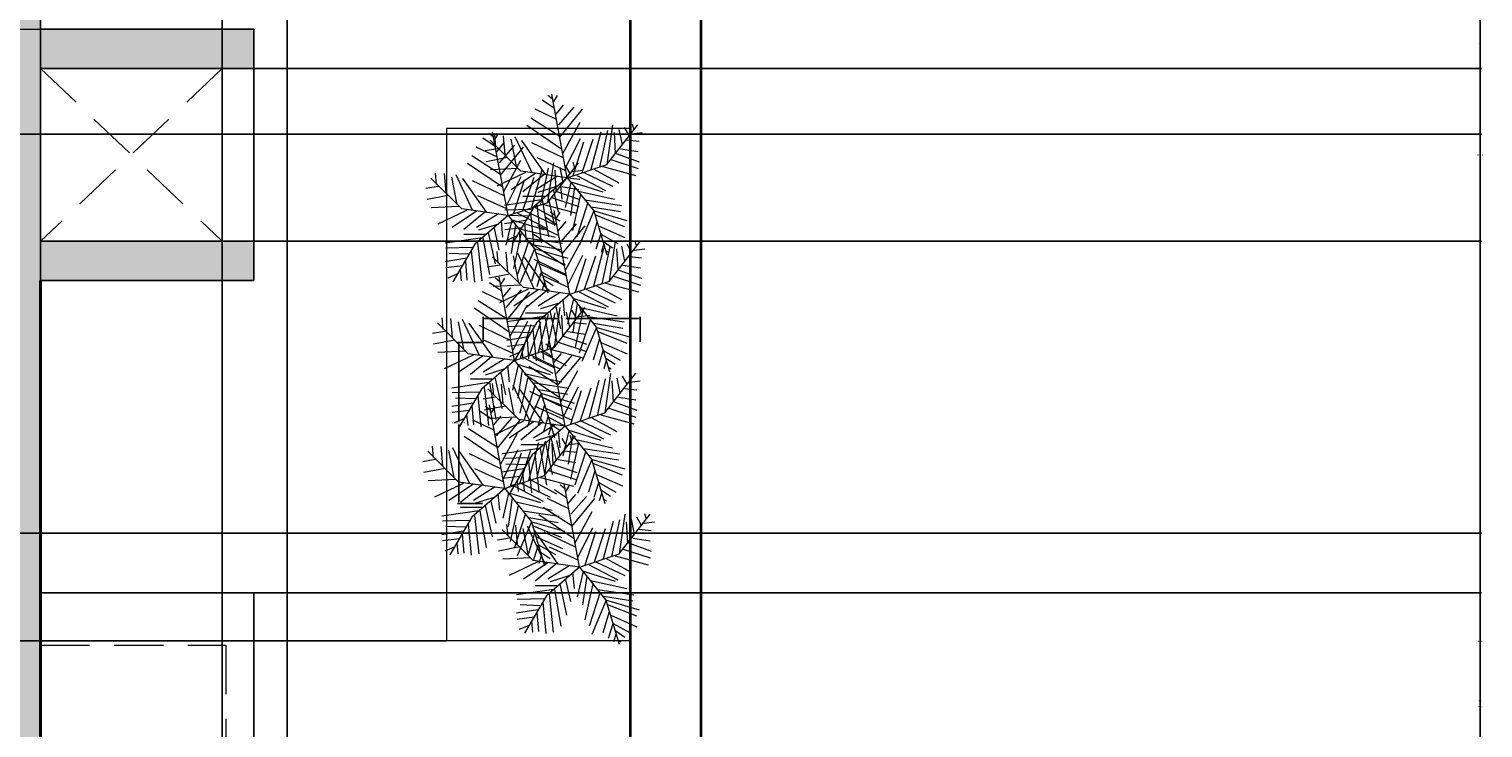
# Model space of a CAD drawing. Units: inches. Extents: x 818 to 1898, y 976 to 2364.
# Tile 92 of 96: x 1713 to 1898, y 1873 to 1962. Entities that reach past the tile are written whole.
import ezdxf

# ---------------------------------------------------------------- set-up
doc = ezdxf.new("R2010")
doc.units = ezdxf.units.IN
doc.header["$LTSCALE"] = 5
doc.header["$MEASUREMENT"] = 0
doc.linetypes.add('HIDDEN', pattern=[0.375, 0.25, -0.125])
for name, color, linetype, lineweight in [('A-ANNO-DIMS', 2, 'Continuous', 18), ('A-FLOR-OVHD', 8, 'HIDDEN', 13), ('A-FLOR-SHFT', 7, 'Continuous', 25), ('A-FLOR-SHFT-HIDN', 8, 'HIDDEN', 13), ('A-FLOR-STRS', 7, 'Continuous', 25), ('A-GLAZ', 4, 'Continuous', 18), ('A-WALL', 7, 'Continuous', 40), ('A-WALL-HIDN', 7, 'HIDDEN', 18), ('C-PROP', 7, 'Continuous', 35), ('L-PLNT-BEDS', 94, 'Continuous', 18)]:
    doc.layers.add(name, color=color, linetype=linetype, lineweight=lineweight)
for name, color, linetype, lineweight, true_color in [('A-GLAZ-PATT', 141, 'Continuous', 9, 0xadddf7), ('A-WALL-PATT', 251, 'Continuous', 13, 0x636466), ('L-PLNT', 116, 'Continuous', 13, 0x136734)]:
    doc.layers.add(name, color=color, linetype=linetype, lineweight=lineweight, true_color=true_color)
doc.styles.get("Standard").update_dxf_attribs({"font": 'arial.ttf'})
doc.dimstyles.get("Standard").update_dxf_attribs({"dimtxt": 0.18, "dimasz": 0.18, "dimexe": 0.18, "dimexo": 0.0625, "dimgap": 0.09, "dimtad": 0, "dimtih": 1, "dimtoh": 1, "dimdec": 4, "dimzin": 0, "dimdsep": 46, "dimtxsty": 'Standard', "dimcen": 0.09, "dimadec": 0, "dimazin": 0, "dimtfac": 1, "dimtdec": 4, "dimtofl": 0, "dimtmove": 0, "dimatfit": 3, "dimfxl": 1, "dimtolj": 1, "dimtzin": 0, "dimarcsym": 0})

# ---------------------------------------------------------------- blocks, each defined once
blk = doc.blocks.new('SHRUB-ACCENT')
for p, q in [((10.44, 9.82), (8.47, 20.47)), ((9.08, 17.24), (6.37, 18.54)), ((8.8, 18.63), (7.25, 19.67)), ((8.53, 19.84), (7.99, 20.28)), ((8.74, 19.5), (9.21, 20.28)), ((9.01, 17.93), (9.96, 19.06)), ((9.35, 16.54), (11.31, 18.8)), ((9.48, 14.98), (12.39, 18.54)), ((9.48, 15.07), (5.82, 17.41)), ((9.89, 12.9), (12.06, 16.89)), ((1.35, 13.77), (1.22, 15.24)), ((2.3, 15.16), (2.51, 12.72)), ((3.79, 15.07), (5.89, 10.55)), ((9.75, 13.42), (5.28, 16.46)), ((10.23, 11.07), (12.12, 14.81)), ((13.48, 10.9), (14.76, 15.68)), ((14.56, 11.16), (15.58, 15.85)), ((15.49, 11.5), (19.41, 16.55)), ((15.51, 11.51), (16.25, 16.54)), ((16.39, 15.59), (16.53, 12.9)), ((17, 15.94), (17.41, 14.03)), ((17.68, 16.2), (18.29, 15.16)), ((18.62, 15.42), (19.98, 15.59)), ((18.69, 16.63), (18.9, 15.94)), ((1.56, 13.51), (0, 13.25)), ((4.55, 10.66), (0.62, 14.58)), ((3.25, 14.72), (3.93, 11.25)), ((7.72, 10.21), (4.67, 14.55)), ((5.89, 14.29), (9.89, 12.38)), ((11.17, 10.12), (12.53, 14.37)), ((12.33, 10.47), (13.75, 14.72)), ((17.2, 13.51), (19.44, 13.16)), ((18.02, 14.63), (19.57, 14.46)), ((2.84, 12.38), (0.14, 11.86)), ((6.57, 12.38), (10.23, 10.73)), ((10.44, 9.82), (15.49, 11.5)), ((14.97, 11.25), (19.17, 10.12)), ((15.98, 12.12), (19.44, 10.99)), ((16.66, 12.9), (19.57, 11.86)), ((4.2, 10.99), (0.68, 10.81)), ((5.15, 10.47), (1.49, 8.73)), ((6.43, 10.38), (3.32, 8.3)), ((10.44, 9.82), (4.55, 10.66)), ((7.45, 10.21), (4.81, 8.04)), ((10.44, 9.82), (6.23, 6.17)), ((9.21, 10.03), (6.43, 8.3)), ((10.9, 9.25), (10.16, 6.04)), ((10.44, 9.82), (13.8, 5.61)), ((10.77, 9.34), (14.97, 8.04)), ((11.65, 10.12), (15.31, 8.21)), ((12.53, 10.47), (16.19, 8.73)), ((13.82, 10.9), (17, 9.16)), ((7.59, 7.43), (4.81, 7.43)), ((9.21, 8.73), (6.7, 7.95)), ((7.92, 7.69), (8.8, 3.69)), ((8.67, 8.21), (9.28, 5.43)), ((9.55, 9.16), (9.75, 7.08)), ((11.38, 8.64), (10.84, 5)), ((12.12, 7.69), (11.11, 3.09)), ((11.85, 8.12), (16.46, 7.08)), ((7.18, 6.99), (2.44, 6.3)), ((5.89, 5.78), (2.51, 5.69)), ((6.23, 6.17), (3.43, 1.4)), ((6.57, 6.39), (7.11, 1.52)), ((7.25, 6.99), (8.06, 2.31)), ((13.07, 6.65), (11.65, 2.31)), ((13.82, 5.6), (11.99, 1.26)), ((12.73, 6.99), (17.34, 6.3)), ((13.48, 6.13), (17.2, 5.52)), ((13.8, 5.61), (15.49, 0)), ((13.88, 5.6), (18.02, 4.39)), ((5.15, 4.39), (2.44, 3.95)), ((5.42, 4.91), (2.91, 5)), ((5.01, 4.04), (5.21, 1.61)), ((5.76, 5.34), (6.16, 1.35)), ((14.22, 4.13), (13.41, 1.44)), ((14.02, 5.08), (17.68, 3.61)), ((4.67, 3.43), (2.51, 3.17)), ((4, 2.39), (2.78, 1.87)), ((4.33, 2.91), (4.47, 1.52)), ((14.7, 2.74), (14.09, 0.74)), ((14.43, 3.69), (17.74, 2.22)), ((14.7, 2.65), (16.86, 1.44)), ((15.04, 1.26), (14.76, 0.31)), ((15.04, 1.7), (16.19, 0.92)), ((15.44, 0.48), (15.71, 0.31))]:
    blk.add_line(p, q)
blk = doc.blocks.new('PLANTER-RECT')
at = {"ltscale": 5}
blk.add_lwpolyline([(23.37, 65.17), (0, 65.17), (0, 0), (23.37, 0)], close=True, dxfattribs=at)
blk = doc.blocks.new('*D24')
at = {"layer": 'A-ANNO-DIMS', "color": 0, "lineweight": -2, "ltscale": 5, "transparency": 16777216}
for p, q in [((1770.93, 1922.15), (1767.74, 1922.15)), ((1767.92, 1921.97), (1767.92, 1912.09)), ((1767.92, 1901.85), (1767.92, 1911.73)), ((1770.93, 1901.67), (1767.74, 1901.67))]:
    blk.add_line(p, q, dxfattribs=at)
at = {"layer": 'A-ANNO-DIMS', "color": 0, "ltscale": 5, "transparency": 16777216}
for points in [[(1767.89, 1921.97), (1767.95, 1921.97), (1767.92, 1922.15)], [(1767.89, 1901.85), (1767.95, 1901.85), (1767.92, 1901.67)]]:
    blk.add_solid(points, dxfattribs=at)
at = {"layer": 'Defpoints', "color": 0, "ltscale": 5, "transparency": 16777216}
for p in [(1767.92, 1922.15), (1770.99, 1922.15), (1770.99, 1901.67)]:
    blk.add_point(p, dxfattribs=at)
at = {"layer": 'A-ANNO-DIMS', "color": 0, "ltscale": 5, "transparency": 16777216, "insert": (1767.92, 1911.91), "char_height": 0.18, "attachment_point": 5}
blk.add_mtext('\\A1;SHRUB 20 TYP.', dxfattribs=at)
blk = doc.blocks.new('*D25')
at = {"layer": 'A-ANNO-DIMS', "color": 0, "lineweight": -2, "ltscale": 5, "transparency": 16777216}
for p, q in [((1770.99, 1922.21), (1770.99, 1925.4)), ((1771.17, 1925.22), (1780.45, 1925.22)), ((1790.79, 1925.22), (1781.51, 1925.22)), ((1790.97, 1922.21), (1790.97, 1925.4))]:
    blk.add_line(p, q, dxfattribs=at)
at = {"layer": 'A-ANNO-DIMS', "color": 0, "ltscale": 5, "transparency": 16777216}
for points in [[(1771.17, 1925.25), (1771.17, 1925.19), (1770.99, 1925.22)], [(1790.79, 1925.25), (1790.79, 1925.19), (1790.97, 1925.22)]]:
    blk.add_solid(points, dxfattribs=at)
at = {"layer": 'Defpoints', "color": 0, "ltscale": 5, "transparency": 16777216}
for p in [(1790.97, 1925.22), (1770.99, 1922.15), (1790.97, 1922.15)]:
    blk.add_point(p, dxfattribs=at)
at = {"layer": 'A-ANNO-DIMS', "color": 0, "ltscale": 5, "transparency": 16777216, "insert": (1780.98, 1925.22), "char_height": 0.18, "attachment_point": 5}
blk.add_mtext('\\A1;20 TYP.', dxfattribs=at)
blk = doc.blocks.new('*D71')
at = {"layer": 'A-ANNO-DIMS', "color": 0, "lineweight": -2, "ltscale": 5, "transparency": 16777216}
for p, q in [((1714.79, 2053.08), (1897.92, 2053.08)), ((1897.74, 2052.9), (1897.74, 1699.76)), ((1897.74, 1346.26), (1897.74, 1699.4)), ((1714.79, 1346.08), (1897.92, 1346.08))]:
    blk.add_line(p, q, dxfattribs=at)
at = {"layer": 'A-ANNO-DIMS', "color": 0, "ltscale": 5, "transparency": 16777216}
for points in [[(1897.71, 2052.9), (1897.77, 2052.9), (1897.74, 2053.08)], [(1897.71, 1346.26), (1897.77, 1346.26), (1897.74, 1346.08)]]:
    blk.add_solid(points, dxfattribs=at)
at = {"layer": 'Defpoints', "color": 0, "ltscale": 5, "transparency": 16777216}
for p in [(1714.73, 2053.08), (1897.74, 2053.08), (1714.73, 1346.08)]:
    blk.add_point(p, dxfattribs=at)
at = {"layer": 'A-ANNO-DIMS', "color": 0, "ltscale": 5, "transparency": 16777216, "insert": (1897.74, 1699.58), "char_height": 0.18, "attachment_point": 5}
blk.add_mtext('\\A1;707', dxfattribs=at)
blk = doc.blocks.new('*D85')
at = {"layer": 'A-ANNO-DIMS', "color": 0, "lineweight": -2, "ltscale": 5, "transparency": 16777216}
for p, q in [((1258.79, 2053.08), (1897.92, 2053.08)), ((1897.74, 2052.9), (1897.74, 1876.76)), ((1897.74, 1700.26), (1897.74, 1876.4)), ((1258.79, 1700.08), (1897.92, 1700.08))]:
    blk.add_line(p, q, dxfattribs=at)
at = {"layer": 'A-ANNO-DIMS', "color": 0, "ltscale": 5, "transparency": 16777216}
for points in [[(1897.71, 2052.9), (1897.77, 2052.9), (1897.74, 2053.08)], [(1897.71, 1700.26), (1897.77, 1700.26), (1897.74, 1700.08)]]:
    blk.add_solid(points, dxfattribs=at)
at = {"layer": 'Defpoints', "color": 0, "ltscale": 5, "transparency": 16777216}
for p in [(1258.73, 2053.08), (1897.74, 2053.08), (1258.73, 1700.08)]:
    blk.add_point(p, dxfattribs=at)
at = {"layer": 'A-ANNO-DIMS', "color": 0, "ltscale": 5, "transparency": 16777216, "insert": (1897.74, 1876.58), "char_height": 0.18, "attachment_point": 5}
blk.add_mtext('\\A1;353', dxfattribs=at)
blk = doc.blocks.new('*D104')
at = {"layer": 'A-ANNO-DIMS', "color": 0, "lineweight": -2, "ltscale": 5, "transparency": 16777216}
for p, q in [((1689.47, 1071.12), (1689.47, 2363.87)), ((1689.65, 2363.69), (1717.4, 2363.69)), ((1745.9, 2363.69), (1718.15, 2363.69)), ((1746.08, 1071.12), (1746.08, 2363.87))]:
    blk.add_line(p, q, dxfattribs=at)
at = {"layer": 'A-ANNO-DIMS', "color": 0, "ltscale": 5, "transparency": 16777216}
for points in [[(1689.65, 2363.72), (1689.65, 2363.66), (1689.47, 2363.69)], [(1745.9, 2363.72), (1745.9, 2363.66), (1746.08, 2363.69)]]:
    blk.add_solid(points, dxfattribs=at)
at = {"layer": 'Defpoints', "color": 0, "ltscale": 5, "transparency": 16777216}
for p in [(1746.08, 2363.69), (1689.47, 1071.06), (1746.08, 1071.06)]:
    blk.add_point(p, dxfattribs=at)
at = {"layer": 'A-ANNO-DIMS', "color": 0, "ltscale": 5, "transparency": 16777216, "insert": (1717.78, 2363.69), "char_height": 0.18, "attachment_point": 5}
blk.add_mtext('\\A1;56.61', dxfattribs=at)
blk = doc.blocks.new('*D121')
at = {"layer": 'A-ANNO-DIMS', "color": 0, "lineweight": -2, "ltscale": 5, "transparency": 16777216}
for p, q in [((1766.29, 1884.2), (818.03, 1884.2)), ((818.21, 1884.02), (818.21, 1841.14)), ((818.21, 1797.9), (818.21, 1840.78)), ((1766.29, 1797.72), (818.03, 1797.72))]:
    blk.add_line(p, q, dxfattribs=at)
at = {"layer": 'A-ANNO-DIMS', "color": 0, "ltscale": 5, "transparency": 16777216}
for points in [[(818.18, 1884.02), (818.24, 1884.02), (818.21, 1884.2)], [(818.18, 1797.9), (818.24, 1797.9), (818.21, 1797.72)]]:
    blk.add_solid(points, dxfattribs=at)
at = {"layer": 'Defpoints', "color": 0, "ltscale": 5, "transparency": 16777216}
for p in [(818.21, 1884.2), (1766.35, 1884.2), (1766.35, 1797.72)]:
    blk.add_point(p, dxfattribs=at)
at = {"layer": 'A-ANNO-DIMS', "color": 0, "ltscale": 5, "transparency": 16777216, "insert": (818.21, 1840.96), "char_height": 0.18, "attachment_point": 5}
blk.add_mtext('\\A1;86.49', dxfattribs=at)
blk = doc.blocks.new('*D186')
at = {"layer": 'A-ANNO-DIMS', "color": 0, "lineweight": -2, "ltscale": 5, "transparency": 16777216}
for p, q in [((1714.73, 1549.14), (1714.73, 2363.87)), ((1714.91, 2363.69), (1725.82, 2363.69)), ((1737.66, 2363.69), (1726.75, 2363.69)), ((1737.84, 1549.14), (1737.84, 2363.87))]:
    blk.add_line(p, q, dxfattribs=at)
at = {"layer": 'A-ANNO-DIMS', "color": 0, "ltscale": 5, "transparency": 16777216}
for points in [[(1714.91, 2363.72), (1714.91, 2363.66), (1714.73, 2363.69)], [(1737.66, 2363.72), (1737.66, 2363.66), (1737.84, 2363.69)]]:
    blk.add_solid(points, dxfattribs=at)
at = {"layer": 'Defpoints', "color": 0, "ltscale": 5, "transparency": 16777216}
for p in [(1737.84, 2363.69), (1714.73, 1549.08), (1737.84, 1549.08)]:
    blk.add_point(p, dxfattribs=at)
at = {"layer": 'A-ANNO-DIMS', "color": 0, "ltscale": 5, "transparency": 16777216, "insert": (1726.28, 2363.69), "char_height": 0.18, "attachment_point": 5}
blk.add_mtext('\\A1;23.116', dxfattribs=at)
blk = doc.blocks.new('*D204')
at = {"layer": 'A-ANNO-DIMS', "color": 0, "lineweight": -2, "ltscale": 5, "transparency": 16777216}
for p, q in [((1714.79, 2053.08), (1897.92, 2053.08)), ((1897.74, 2052.9), (1897.74, 1960.26)), ((1897.74, 1867.26), (1897.74, 1959.9)), ((1705.79, 1867.08), (1897.92, 1867.08))]:
    blk.add_line(p, q, dxfattribs=at)
at = {"layer": 'A-ANNO-DIMS', "color": 0, "ltscale": 5, "transparency": 16777216}
for points in [[(1897.71, 2052.9), (1897.77, 2052.9), (1897.74, 2053.08)], [(1897.71, 1867.26), (1897.77, 1867.26), (1897.74, 1867.08)]]:
    blk.add_solid(points, dxfattribs=at)
at = {"layer": 'Defpoints', "color": 0, "ltscale": 5, "transparency": 16777216}
for p in [(1714.73, 2053.08), (1897.74, 2053.08), (1705.73, 1867.08)]:
    blk.add_point(p, dxfattribs=at)
at = {"layer": 'A-ANNO-DIMS', "color": 0, "ltscale": 5, "transparency": 16777216, "insert": (1897.74, 1960.08), "char_height": 0.18, "attachment_point": 5}
blk.add_mtext('\\A1;186', dxfattribs=at)
blk = doc.blocks.new('*D239')
at = {"layer": 'A-ANNO-DIMS', "color": 0, "lineweight": -2, "ltscale": 5, "transparency": 16777216}
for p, q in [((1483.61, 1979.24), (1897.92, 1979.24)), ((1897.74, 1979.06), (1897.74, 1964.13)), ((1897.74, 1948.84), (1897.74, 1963.77)), ((1483.61, 1948.66), (1897.92, 1948.66))]:
    blk.add_line(p, q, dxfattribs=at)
at = {"layer": 'A-ANNO-DIMS', "color": 0, "ltscale": 5, "transparency": 16777216}
for points in [[(1897.71, 1979.06), (1897.77, 1979.06), (1897.74, 1979.24)], [(1897.71, 1948.84), (1897.77, 1948.84), (1897.74, 1948.66)]]:
    blk.add_solid(points, dxfattribs=at)
at = {"layer": 'Defpoints', "color": 0, "ltscale": 5, "transparency": 16777216}
for p in [(1483.55, 1979.24), (1897.74, 1979.24), (1483.55, 1948.66)]:
    blk.add_point(p, dxfattribs=at)
at = {"layer": 'A-ANNO-DIMS', "color": 0, "ltscale": 5, "transparency": 16777216, "insert": (1897.74, 1963.95), "char_height": 0.18, "attachment_point": 5}
blk.add_mtext('\\A1;30.584', dxfattribs=at)
blk = doc.blocks.new('*D262')
at = {"layer": 'A-ANNO-DIMS', "color": 0, "lineweight": -2, "ltscale": 5, "transparency": 16777216}
for p, q in [((1714.73, 1957.1), (1714.73, 2363.87)), ((1714.91, 2363.69), (1725.82, 2363.69)), ((1737.66, 2363.69), (1726.75, 2363.69)), ((1737.84, 1957.1), (1737.84, 2363.87))]:
    blk.add_line(p, q, dxfattribs=at)
at = {"layer": 'A-ANNO-DIMS', "color": 0, "ltscale": 5, "transparency": 16777216}
for points in [[(1714.91, 2363.72), (1714.91, 2363.66), (1714.73, 2363.69)], [(1737.66, 2363.72), (1737.66, 2363.66), (1737.84, 2363.69)]]:
    blk.add_solid(points, dxfattribs=at)
at = {"layer": 'Defpoints', "color": 0, "ltscale": 5, "transparency": 16777216}
for p in [(1737.84, 2363.69), (1714.73, 1957.03), (1737.84, 1957.03)]:
    blk.add_point(p, dxfattribs=at)
at = {"layer": 'A-ANNO-DIMS', "color": 0, "ltscale": 5, "transparency": 16777216, "insert": (1726.28, 2363.69), "char_height": 0.18, "attachment_point": 5}
blk.add_mtext('\\A1;23.116', dxfattribs=at)
blk = doc.blocks.new('*D263')
at = {"layer": 'A-ANNO-DIMS', "color": 0, "lineweight": -2, "ltscale": 5, "transparency": 16777216}
for p, q in [((1737.9, 1957.03), (1897.92, 1957.03)), ((1897.74, 1956.85), (1897.74, 1946.21)), ((1897.74, 1935.21), (1897.74, 1945.85)), ((1737.9, 1935.03), (1897.92, 1935.03))]:
    blk.add_line(p, q, dxfattribs=at)
at = {"layer": 'A-ANNO-DIMS', "color": 0, "ltscale": 5, "transparency": 16777216}
for points in [[(1897.71, 1956.85), (1897.77, 1956.85), (1897.74, 1957.03)], [(1897.71, 1935.21), (1897.77, 1935.21), (1897.74, 1935.03)]]:
    blk.add_solid(points, dxfattribs=at)
at = {"layer": 'Defpoints', "color": 0, "ltscale": 5, "transparency": 16777216}
for p in [(1737.84, 1957.03), (1897.74, 1957.03), (1737.84, 1935.03)]:
    blk.add_point(p, dxfattribs=at)
at = {"layer": 'A-ANNO-DIMS', "color": 0, "ltscale": 5, "transparency": 16777216, "insert": (1897.74, 1946.03), "char_height": 0.18, "attachment_point": 5}
blk.add_mtext('\\A1;22.002', dxfattribs=at)
blk = doc.blocks.new('*D268')
at = {"layer": 'A-ANNO-DIMS', "color": 0, "lineweight": -2, "ltscale": 5, "transparency": 16777216}
for p, q in [((1741.9, 1890.29), (1897.92, 1890.29)), ((1897.74, 1890.11), (1897.74, 1788.87)), ((1897.74, 1687.26), (1897.74, 1788.5)), ((1741.9, 1687.08), (1897.92, 1687.08))]:
    blk.add_line(p, q, dxfattribs=at)
at = {"layer": 'A-ANNO-DIMS', "color": 0, "ltscale": 5, "transparency": 16777216}
for points in [[(1897.71, 1890.11), (1897.77, 1890.11), (1897.74, 1890.29)], [(1897.71, 1687.26), (1897.77, 1687.26), (1897.74, 1687.08)]]:
    blk.add_solid(points, dxfattribs=at)
at = {"layer": 'Defpoints', "color": 0, "ltscale": 5, "transparency": 16777216}
for p in [(1741.84, 1890.29), (1897.74, 1890.29), (1741.84, 1687.08)]:
    blk.add_point(p, dxfattribs=at)
at = {"layer": 'A-ANNO-DIMS', "color": 0, "ltscale": 5, "transparency": 16777216, "insert": (1897.74, 1788.68), "char_height": 0.18, "attachment_point": 5}
blk.add_mtext('\\A1;203.2', dxfattribs=at)
blk = doc.blocks.new('*D275')
at = {"layer": 'A-ANNO-DIMS', "color": 0, "lineweight": -2, "ltscale": 5, "transparency": 16777216}
for p, q in [((1377.84, 1897.87), (1897.92, 1897.87)), ((1897.74, 1897.69), (1897.74, 1875.99)), ((1897.74, 1853.93), (1897.74, 1875.63)), ((1377.84, 1853.75), (1897.92, 1853.75))]:
    blk.add_line(p, q, dxfattribs=at)
at = {"layer": 'A-ANNO-DIMS', "color": 0, "ltscale": 5, "transparency": 16777216}
for points in [[(1897.71, 1897.69), (1897.77, 1897.69), (1897.74, 1897.87)], [(1897.71, 1853.93), (1897.77, 1853.93), (1897.74, 1853.75)]]:
    blk.add_solid(points, dxfattribs=at)
at = {"layer": 'Defpoints', "color": 0, "ltscale": 5, "transparency": 16777216}
for p in [(1377.78, 1897.87), (1897.74, 1897.87), (1377.78, 1853.75)]:
    blk.add_point(p, dxfattribs=at)
at = {"layer": 'A-ANNO-DIMS', "color": 0, "ltscale": 5, "transparency": 16777216, "insert": (1897.74, 1875.81), "char_height": 0.18, "attachment_point": 5}
blk.add_mtext('\\A1;44.12', dxfattribs=at)
blk = doc.blocks.new('*D282')
at = {"layer": 'A-ANNO-DIMS', "color": 0, "lineweight": -2, "ltscale": 5, "transparency": 16777216}
for p, q in [((1422.08, 2081.19), (1897.92, 2081.19)), ((1897.74, 2081.01), (1897.74, 1884.32)), ((1897.74, 1687.26), (1897.74, 1883.95)), ((1463.79, 1687.08), (1897.92, 1687.08))]:
    blk.add_line(p, q, dxfattribs=at)
at = {"layer": 'A-ANNO-DIMS', "color": 0, "ltscale": 5, "transparency": 16777216}
for points in [[(1897.71, 2081.01), (1897.77, 2081.01), (1897.74, 2081.19)], [(1897.71, 1687.26), (1897.77, 1687.26), (1897.74, 1687.08)]]:
    blk.add_solid(points, dxfattribs=at)
at = {"layer": 'Defpoints', "color": 0, "ltscale": 5, "transparency": 16777216}
for p in [(1422.02, 2081.19), (1897.74, 2081.19), (1463.73, 1687.08)]:
    blk.add_point(p, dxfattribs=at)
at = {"layer": 'A-ANNO-DIMS', "color": 0, "ltscale": 5, "transparency": 16777216, "insert": (1897.74, 1884.13), "char_height": 0.18, "attachment_point": 5}
blk.add_mtext('\\A1;394.1', dxfattribs=at)

msp = doc.modelspace()

# ---------------------------------------------------------------- hatches: boundary and pattern name
at = {"layer": 'A-GLAZ-PATT', "ltscale": 5}
h = msp.add_hatch(color=256, dxfattribs=at)
h.dxf.hatch_style = 1
h.paths.add_polyline_path([(1283.8183, 1504.5782), (1206.7252, 1504.5782), (1206.7252, 1501.0782), (1283.8183, 1501.0782)])
h.paths.add_polyline_path([(1283.8183, 1510.0782), (1206.7252, 1510.0782), (1206.7252, 1506.5782), (1283.8183, 1506.5782)])
h.paths.add_polyline_path([(1490.9163, 1355.0782), (1439.7252, 1355.0782), (1439.7252, 1409.0522), (1436.2252, 1409.0522), (1436.2252, 1351.5782), (1490.9163, 1351.5782)])
h.paths.add_polyline_path([(1434.2252, 1409.0522), (1430.7252, 1409.0522), (1430.7252, 1346.0782), (1435.0799, 1346.0782), (1435.0731, 1346.1152), (1435.1501, 1346.0782), (1490.9163, 1346.0782), (1490.9163, 1349.5782), (1434.2252, 1349.5782)])
h.paths.add_polyline_path([(1714.7251, 1545.0782), (1711.2252, 1545.0782), (1711.2252, 1521.0782), (1714.7251, 1521.0782)])
h.paths.add_polyline_path([(1709.2252, 1545.0782), (1705.7251, 1545.0782), (1705.7251, 1521.0782), (1709.2252, 1521.0782)])
h.paths.add_polyline_path([(1714.7251, 1687.0782), (1711.2252, 1687.0782), (1711.2252, 1649.9029), (1714.7251, 1649.9029)])
h.paths.add_polyline_path([(1709.2252, 1687.0782), (1705.7251, 1687.0782), (1705.7251, 1649.9029), (1709.2252, 1649.9029)])
h.paths.add_polyline_path([(1709.2252, 1745.5584), (1705.7251, 1745.5584), (1705.7251, 1717.3178), (1709.2252, 1717.3178)])
h.paths.add_polyline_path([(1714.7251, 1745.5584), (1711.2252, 1745.5584), (1711.2252, 1717.3178), (1714.7251, 1717.3178)])
h.paths.add_polyline_path([(1714.7251, 2014.5114), (1711.2252, 2014.5114), (1711.2252, 1962.0338), (1714.7251, 1962.0338)])
h.paths.add_polyline_path([(1709.2252, 2014.5114), (1705.7251, 2014.5114), (1705.7251, 1962.0338), (1709.2252, 1962.0338)])
h.paths.add_polyline_path([(1538.5155, 2047.5782), (1485.1216, 2047.5782), (1485.1216, 2044.0782), (1538.5155, 2044.0782)])
h.paths.add_polyline_path([(1538.5155, 2053.0782), (1485.1216, 2053.0782), (1485.1216, 2049.5782), (1538.5155, 2049.5782)])
h.paths.add_polyline_path([(1388.0315, 2047.5782), (1330.305, 2047.5782), (1330.305, 2044.0782), (1388.0315, 2044.0782)])
h.paths.add_polyline_path([(1388.0315, 2053.0782), (1330.305, 2053.0782), (1330.305, 2049.5782), (1388.0315, 2049.5782)])
h.paths.add_polyline_path([(1262.2252, 2019.2871), (1258.7251, 2019.2871), (1258.7251, 1928.9218), (1262.2252, 1928.9218)])
h.paths.add_polyline_path([(1267.7252, 2019.2871), (1264.2252, 2019.2871), (1264.2252, 1928.9218), (1267.7252, 1928.9218)])
h.paths.add_polyline_path([(1262.2252, 1862.9652), (1258.7251, 1862.9652), (1258.7251, 1814.9652), (1262.2252, 1814.9652)])
h.paths.add_polyline_path([(1267.7252, 1862.9652), (1264.2252, 1862.9652), (1264.2252, 1814.9652), (1267.7252, 1814.9652)])
h.paths.add_polyline_path([(1262.2252, 1755.3321), (1258.7251, 1755.3321), (1258.7251, 1707.3321), (1262.2252, 1707.3321)])
h.paths.add_polyline_path([(1267.7252, 1755.3321), (1264.2252, 1755.3321), (1264.2252, 1707.3321), (1267.7252, 1707.3321)])
h.paths.add_polyline_path([(1251.9333, 1692.5782), (1206.7252, 1692.5782), (1206.7252, 1687.0782), (1251.9333, 1687.0782)])
h.paths.add_polyline_path([(1251.9333, 1700.0782), (1206.7252, 1700.0782), (1206.7252, 1694.5782), (1251.9333, 1694.5782)])
at = {"layer": 'A-WALL-PATT', "ltscale": 5}
h = msp.add_hatch(color=256, dxfattribs=at)
h.dxf.hatch_style = 1
h.paths.add_polyline_path([(1267.7252, 1928.9218), (1258.7251, 1928.9218), (1258.7251, 1913.6401), (1250.3029, 1913.6401), (1250.3029, 1878.3919), (1258.7251, 1878.3919), (1258.7251, 1862.9652), (1267.7252, 1862.9652)])
h.paths.add_polyline_path([(1267.7252, 1814.9652), (1258.7251, 1814.9652), (1258.7251, 1755.3321), (1267.7252, 1755.3321)])
h.paths.add_polyline_path([(1463.7251, 1696.0782), (1267.7252, 1696.0782), (1267.7252, 1707.3321), (1258.7251, 1707.3321), (1258.7251, 1700.0782), (1251.9333, 1700.0782), (1251.9333, 1687.0782), (1463.7251, 1687.0782)])
h.paths.add_polyline_path([(1714.7251, 1717.3178), (1705.7251, 1717.3178), (1705.7251, 1696.0782), (1599.7252, 1696.0782), (1599.7252, 1790.0782), (1705.7251, 1790.0782), (1705.7251, 1785.6125), (1714.7251, 1785.6125), (1714.7251, 1827.2125), (1705.7251, 1827.2125), (1705.7251, 1802.0782), (1599.7252, 1802.0782), (1599.7252, 1867.0782), (1705.7251, 1867.0782), (1705.7251, 1857.2125), (1714.7251, 1857.2125), (1714.7251, 1930.0316), (1741.8409, 1930.0316), (1741.8409, 1935.0316), (1714.7251, 1935.0316), (1714.7251, 1957.0338), (1741.8409, 1957.0338), (1741.8409, 1962.0338), (1714.7251, 1962.0338), (1705.7251, 1962.0338), (1705.7251, 1948.0782), (1599.7252, 1948.0782), (1599.7252, 1981.0782), (1590.7252, 1981.0782), (1590.7252, 1941.0782), (1620.7252, 1941.0782), (1705.7251, 1941.0782), (1705.7251, 1876.0782), (1599.7252, 1876.0782), (1599.7252, 1911.0782), (1590.7252, 1911.0782), (1590.7252, 1876.0782), (1429.2252, 1876.0782), (1429.2252, 1867.0782), (1511.7252, 1867.0782), (1528.593, 1867.0782), (1595.7252, 1867.0782), (1595.7252, 1773.0782), (1520.7252, 1773.0782), (1520.7252, 1837.5823), (1532.593, 1837.5823), (1532.593, 1867.0782), (1528.593, 1867.0782), (1528.593, 1841.5823), (1511.7252, 1841.5823), (1511.7252, 1744.9714), (1520.7252, 1744.9714), (1520.7252, 1761.0782), (1595.7252, 1761.0782), (1595.7252, 1696.0782), (1520.7252, 1696.0782), (1520.7252, 1716.0454), (1511.7252, 1716.0454), (1511.7252, 1696.0782), (1511.7252, 1687.0782), (1714.7251, 1687.0782)])
h.paths.add_polyline_path([(1714.7251, 2053.0782), (1714.7251, 2081.1881), (1709.7252, 2081.1881), (1709.7252, 2053.0782), (1681.6446, 2053.0782), (1681.6446, 2081.1881), (1676.6446, 2081.1881), (1676.6446, 2053.0782), (1538.5155, 2053.0782), (1538.5155, 2044.0782), (1590.7252, 2044.0782), (1590.7252, 2011.0782), (1599.7252, 2011.0782), (1599.7252, 2044.0782), (1705.7251, 2044.0782), (1705.7251, 2014.5114), (1714.7251, 2014.5114)])
h.paths.add_polyline_path([(1485.1216, 2053.0782), (1422.02, 2053.0782), (1422.02, 2081.1881), (1413.02, 2081.1881), (1413.02, 2053.0782), (1399.6356, 2053.0782), (1399.6356, 2081.1881), (1390.6356, 2081.1881), (1390.6356, 2053.0782), (1388.0315, 2053.0782), (1388.0315, 2044.0782), (1416.2743, 2044.0782), (1485.1216, 2044.0782)])
h.paths.add_polyline_path([(1330.305, 2053.0782), (1258.7251, 2053.0782), (1258.7251, 2019.2871), (1267.7252, 2019.2871), (1267.7252, 2044.0782), (1330.305, 2044.0782)])
h.paths.add_polyline_path([(1258.7251, 2053.0782), (1214.6577, 2053.0782), (1214.6577, 2044.0782), (1258.7251, 2044.0782)])
h.paths.add_polyline_path([(1214.6577, 2053.0782), (1180.349, 2053.0782), (1180.349, 2044.0782), (1214.6577, 2044.0782)])
h.paths.add_polyline_path([(1714.7251, 1639.5782), (1741.8409, 1639.5782), (1741.8409, 1643.5782), (1714.7251, 1643.5782), (1714.7251, 1649.9029), (1705.7251, 1649.9029), (1705.7251, 1600.0782), (1477.7252, 1600.0782), (1477.7252, 1591.0782), (1520.7252, 1591.0782), (1616.7252, 1591.0782), (1616.7252, 1416.6857), (1622.7252, 1416.6857), (1622.7252, 1463.0782), (1624.7252, 1463.0782), (1624.7252, 1467.0782), (1622.7252, 1467.0782), (1622.7252, 1591.0782), (1705.7251, 1591.0782), (1705.7251, 1545.0782), (1714.7251, 1545.0782), (1741.8409, 1545.0782), (1741.8409, 1549.0782), (1714.7251, 1549.0782), (1714.7251, 1593.9175), (1737.8409, 1593.9175), (1737.8409, 1597.9175), (1714.7251, 1597.9175)])
h.paths.add_polyline_path([(1674.9024, 2060.7419), (1714.7045, 2060.7419), (1714.7045, 2073.1061), (1674.9024, 2073.1061)], flags=25)
h.paths.add_polyline_path([(1394.5468, 2061.6618), (1422.2344, 2061.6618), (1422.2344, 2074.0261), (1394.5468, 2074.0261)], flags=24)

# ---------------------------------------------------------------- linework, layer by layer
at = {"layer": 'A-FLOR-OVHD', "ltscale": 5}
for p, q in [((1714.7251, 1883.6351), (1738.3002, 1883.6351)), ((1738.3002, 1883.6351), (1738.3002, 1692.5441))]:
    msp.add_line(p, q, dxfattribs=at)
at = {"layer": 'A-FLOR-SHFT'}
for p, q in [((1714.7251, 1962.0338), (1741.8409, 1962.0338)), ((1741.8409, 1962.0338), (1741.8409, 1930.0316)), ((1714.7251, 1957.0338), (1741.8409, 1957.0338)), ((1714.7251, 1957.0338), (1714.7251, 1935.0316)), ((1737.8409, 1957.0338), (1737.8409, 1935.0316)), ((1714.7251, 1935.0316), (1741.8409, 1935.0316)), ((1714.7251, 1930.0316), (1741.8409, 1930.0316))]:
    msp.add_line(p, q, dxfattribs=at)
at = {"layer": 'A-FLOR-SHFT-HIDN', "ltscale": 5}
for p, q in [((1737.8409, 1957.0338), (1714.7251, 1935.0316)), ((1714.7251, 1957.0338), (1737.8409, 1935.0316))]:
    msp.add_line(p, q, dxfattribs=at)
at = {"layer": 'A-FLOR-STRS'}
for p, q in [((1714.7251, 1890.2903), (1741.8409, 1890.2903)), ((1741.8409, 1890.2903), (1741.8409, 1759.6099))]:
    msp.add_line(p, q, dxfattribs=at)
at = {"layer": 'A-GLAZ'}
msp.add_line((1705.7251, 1962.0338), (1714.7251, 1962.0338), dxfattribs=at)
at = {"layer": 'A-WALL'}
msp.add_line((1714.7251, 1930.0316), (1714.7251, 1857.2125), dxfattribs=at)
at = {"layer": 'A-WALL-HIDN', "ltscale": 5}
msp.add_line((1714.7355, 2013.5614), (1714.7355, 1962.0338), dxfattribs=at)
at = {"layer": 'C-PROP', "ltscale": 5}
for p, q in [((1798.7173, 1202.9642), (1798.7173, 2294.2171)), ((1789.7173, 1211.9642), (1789.7173, 2285.2171))]:
    msp.add_line(p, q, dxfattribs=at)

# ---------------------------------------------------------------- block references
at = {"layer": 'L-PLNT'}
for p in [(1771.257, 1933.293), (1763.7314, 1928.4742), (1771.5761, 1918.4661), (1764.5652, 1910.053), (1770.9913, 1901.6743), (1763.3302, 1893.7297), (1772.8128, 1883.7438)]:
    msp.add_blockref('SHRUB-ACCENT', p, dxfattribs=at)
at = {"layer": 'L-PLNT-BEDS'}
msp.add_blockref('PLANTER-RECT', (1766.352, 1884.203), dxfattribs=at)

# ---------------------------------------------------------------- dimensions: what is measured, and where the dimension line sits
at = {"layer": 'A-ANNO-DIMS', "ltscale": 5}
for base, p1, p2, override, picture, middle in [((1746.0831, 2363.6929), (1689.4714, 1071.0552), (1746.0831, 1071.0552), {"dimdec": 2, "dimlfac": 1, "dimrnd": 0, "dimzin": 0, "dimdsep": 46, "dimlunit": 2}, '*D104', (1717.7772, 2363.6929)), ((1737.8409, 2363.6929), (1714.7251, 1549.0782), (1737.8409, 1549.0782), {"dimdec": 3, "dimlfac": 1, "dimrnd": 0, "dimzin": 0, "dimdsep": 46, "dimlunit": 2}, '*D186', (1726.283, 2363.6929)), ((1737.8409, 2363.6929), (1714.7251, 1957.0338), (1737.8409, 1957.0338), {"dimdec": 3, "dimlfac": 1, "dimrnd": 0, "dimzin": 0, "dimdsep": 46, "dimlunit": 2}, '*D262', (1726.283, 2363.6929))]:
    dim = msp.add_linear_dim(base=base, p1=p1, p2=p2, dimstyle='Standard', override=override, dxfattribs=at)
    dim.commit()
    dim.dimension.update_dxf_attribs({"geometry": picture, "text_midpoint": middle})
for base, p1, p2, override, picture, middle in [((1897.736, 2081.1881), (1463.7251, 1687.0782), (1422.02, 2081.1881), {"dimdec": 1, "dimlfac": 1, "dimrnd": 0, "dimzin": 0, "dimdsep": 46, "dimlunit": 2}, '*D282', (1897.736, 1884.1332)), ((1897.736, 2053.0782), (1258.7251, 1700.0782), (1258.7251, 2053.0782), {"dimdec": 0, "dimlfac": 1, "dimrnd": 0, "dimzin": 0, "dimdsep": 46, "dimlunit": 2}, '*D85', (1897.736, 1876.5782)), ((1897.736, 2053.0782), (1705.7251, 1867.0782), (1714.7251, 2053.0782), {"dimdec": 0, "dimlfac": 1, "dimrnd": 0, "dimzin": 0, "dimdsep": 46, "dimlunit": 2}, '*D204', (1897.736, 1960.0782)), ((1897.736, 2053.0782), (1714.7251, 1346.0782), (1714.7251, 2053.0782), {"dimdec": 0, "dimlfac": 1, "dimrnd": 0, "dimzin": 0, "dimdsep": 46, "dimlunit": 2}, '*D71', (1897.736, 1699.5782)), ((1897.736, 1979.2444), (1483.5451, 1948.6602), (1483.5451, 1979.2444), {"dimdec": 3, "dimlfac": 1, "dimrnd": 0, "dimzin": 0, "dimdsep": 46, "dimlunit": 2}, '*D239', (1897.736, 1963.9523)), ((1897.736, 1957.0338), (1737.8409, 1935.0316), (1737.8409, 1957.0338), {"dimdec": 3, "dimlfac": 1, "dimrnd": 0, "dimzin": 0, "dimdsep": 46, "dimlunit": 2}, '*D263', (1897.736, 1946.0327)), ((1897.736, 1897.8663), (1377.7791, 1853.7496), (1377.7791, 1897.8663), {"dimdec": 2, "dimlfac": 1, "dimrnd": 0, "dimzin": 0, "dimdsep": 46, "dimlunit": 2}, '*D275', (1897.736, 1875.808)), ((1897.736, 1890.2903), (1741.8409, 1687.0782), (1741.8409, 1890.2903), {"dimdec": 1, "dimlfac": 1, "dimrnd": 0, "dimzin": 0, "dimdsep": 46, "dimlunit": 2}, '*D268', (1897.736, 1788.6843)), ((818.2059, 1884.2031), (1766.3524, 1797.7165), (1766.3524, 1884.2031), {"dimdec": 2, "dimlfac": 1, "dimrnd": 0, "dimzin": 0, "dimdsep": 46, "dimlunit": 2}, '*D121', (818.2059, 1840.9598))]:
    dim = msp.add_linear_dim(base=base, p1=p1, p2=p2, angle=90, dimstyle='Standard', override=override, dxfattribs=at)
    dim.commit()
    dim.dimension.update_dxf_attribs({"geometry": picture, "text_midpoint": middle})
dim = msp.add_linear_dim(base=(1790.9707, 1925.2171), p1=(1770.9913, 1922.1463), p2=(1790.9707, 1922.1463), text='<> TYP.', dimstyle='Standard', override={"dimdec": 0, "dimlfac": 1, "dimrnd": 0, "dimzin": 0, "dimdsep": 46, "dimlunit": 2}, dxfattribs=at)
dim.commit()
dim.dimension.update_dxf_attribs({"geometry": '*D25', "text_midpoint": (1780.981, 1925.2171)})
dim = msp.add_linear_dim(base=(1767.9205, 1922.1463), p1=(1770.9913, 1901.6745), p2=(1770.9913, 1922.1463), angle=90, text='SHRUB <> TYP.', dimstyle='Standard', override={"dimdec": 0, "dimlfac": 1, "dimrnd": 0, "dimzin": 0, "dimdsep": 46, "dimlunit": 2}, dxfattribs=at)
dim.commit()
dim.dimension.update_dxf_attribs({"geometry": '*D24', "text_midpoint": (1767.9205, 1911.9104)})

doc.saveas('drawing.dxf')
